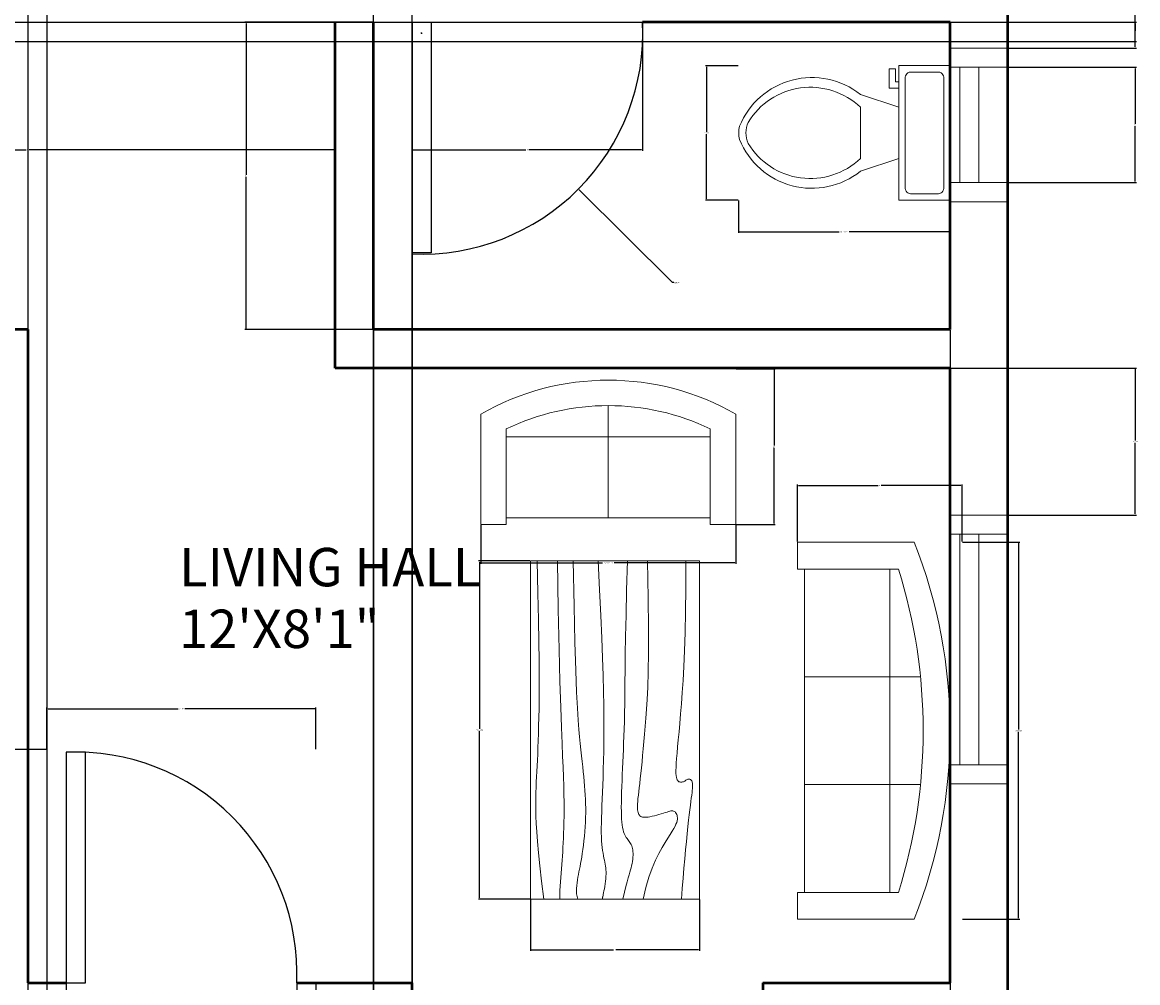
# Model space of a CAD drawing. Units: inches. Extents: x 2630 to 2982, y 643 to 1079.
# Tile 3 of 4: x 2808 to 2982, y 774 to 924. Entities that reach past the tile are written whole.
import ezdxf

# ---------------------------------------------------------------- set-up
doc = ezdxf.new("R2010")
doc.units = ezdxf.units.IN
for name, color, linetype, lineweight in [('A-ANNO-DIMS', 2, 'Continuous', 18), ('A-AREA-IDEN', 7, 'Continuous', 25), ('A-DOOR', 3, 'Continuous', 25), ('A-FLOR-FIXT', 9, 'Continuous', 18), ('A-FURN', 8, 'Continuous', 18), ('A-GLAZ', 4, 'Continuous', 18), ('A-WALL', 7, 'Continuous', 50)]:
    doc.layers.add(name, color=color, linetype=linetype, lineweight=lineweight)
doc.styles.get("Standard").update_dxf_attribs({"font": 'arial.ttf'})
doc.dimstyles.get("Standard").update_dxf_attribs({"dimtxt": 0.18, "dimasz": 0.18, "dimexe": 0.18, "dimexo": 0.0625, "dimgap": 0.09, "dimtad": 0, "dimtih": 1, "dimtoh": 1, "dimdec": 4, "dimzin": 0, "dimdsep": 46, "dimtxsty": 'Standard', "dimcen": 0.09, "dimadec": 0, "dimazin": 0, "dimtfac": 1, "dimtdec": 4, "dimtofl": 0, "dimtmove": 0, "dimatfit": 3, "dimfxl": 1, "dimtolj": 1, "dimtzin": 0, "dimarcsym": 0})

# ---------------------------------------------------------------- blocks, each defined once
blk = doc.blocks.new('Table - Rectangular Woodgrain 60 x 30 in.')
for p, q in [((0, 0), (0, -30)), ((60, 0), (0, 0)), ((60, -30), (60, 0)), ((0, -30), (60, -30))]:
    blk.add_line(p, q)
for points in [[(0, -2.4), (4.8155, -2.418), (9.0302, -2.4688), (12.709, -2.5477), (15.9167, -2.65), (18.7181, -2.7711), (21.1781, -2.9063), (23.3616, -3.0508), (25.3333, -3.2), (27.1477, -3.3495), (28.8172, -3.4958), (30.3437, -3.636), (31.7291, -3.7667), (32.9756, -3.8849), (34.0849, -3.9875), (35.059, -4.0714), (35.9, -4.1334), (36.6114, -4.1711), (37.2041, -4.1854), (37.6906, -4.1779), (38.0833, -4.15), (38.3948, -4.1034), (38.6375, -4.0396), (38.8239, -3.9602), (38.9666, -3.8667), (39.0764, -3.7608), (39.1573, -3.6448), (39.2116, -3.521), (39.2416, -3.3917), (39.2498, -3.2593), (39.2385, -3.1261), (39.21, -2.9944), (39.1666, -2.8667), (39.111, -2.7447), (39.0468, -2.6281), (38.978, -2.5163), (38.9083, -2.4083), (38.8418, -2.3035), (38.7823, -2.201), (38.7337, -2.1001), (38.7, -2), (38.6844, -1.9003), (38.6875, -1.8021), (38.7094, -1.707), (38.75, -1.6167), (38.8094, -1.5326), (38.8875, -1.4563), (38.9844, -1.3893), (39.1, -1.3333), (39.2351, -1.2896), (39.3937, -1.2583), (39.5804, -1.2396), (39.8, -1.2333), (40.057, -1.2396), (40.3562, -1.2583), (40.7023, -1.2896), (41.1, -1.3333), (41.5547, -1.3895), (42.0755, -1.4573), (42.6721, -1.5361), (43.3542, -1.625), (44.1316, -1.7233), (45.014, -1.8302), (46.0114, -1.9449), (47.1333, -2.0667), (48.3862, -2.1947), (49.7625, -2.3281), (51.2513, -2.4663), (52.8416, -2.6083), (54.5226, -2.7535), (56.2833, -2.9011), (58.1127, -3.0501), (60, -3.2)], [(0, -9.2), (6.5759, -9.0858), (11.9385, -9.0365), (16.2527, -9.0418), (19.6833, -9.0917), (22.3952, -9.1759), (24.5531, -9.2844), (26.322, -9.4069), (27.8666, -9.5333), (29.3241, -9.6553), (30.7203, -9.7719), (32.0532, -9.8837), (33.3208, -9.9917), (34.5213, -10.0965), (35.6526, -10.199), (36.7128, -10.2999), (37.7, -10.4), (38.6129, -10.4996), (39.4531, -10.5969), (40.223, -10.6895), (40.925, -10.775), (41.5613, -10.8512), (42.1344, -10.9156), (42.6465, -10.966), (43.1, -11), (43.4976, -11.0158), (43.8437, -11.0136), (44.143, -10.9942), (44.4, -10.9583), (44.6195, -10.9069), (44.8062, -10.8406), (44.9648, -10.7603), (45.1, -10.6667), (45.2155, -10.5598), (45.3114, -10.4365), (45.3871, -10.2929), (45.4416, -10.125), (45.4743, -9.929), (45.4844, -9.7011), (45.4709, -9.4371), (45.4333, -9.1333), (45.3716, -8.7883), (45.2896, -8.4104), (45.1919, -8.0107), (45.0833, -7.6), (44.9685, -7.1893), (44.8521, -6.7896), (44.7388, -6.4117), (44.6333, -6.0667), (44.54, -5.7628), (44.4614, -5.4979), (44.4001, -5.2675), (44.3583, -5.0667), (44.3384, -4.8909), (44.3427, -4.7354), (44.3736, -4.5956), (44.4333, -4.4667), (44.5236, -4.3453), (44.6427, -4.2333), (44.7884, -4.1339), (44.9583, -4.05), (45.1501, -3.9849), (45.3614, -3.9417), (45.59, -3.9234), (45.8333, -3.9333), (46.0915, -3.9749), (46.3734, -4.0531), (46.6906, -4.1736), (47.0542, -4.3417), (47.4756, -4.5629), (47.9661, -4.8427), (48.5372, -5.1866), (49.2, -5.6), (49.9676, -6.0844), (50.8594, -6.625), (51.8965, -7.2031), (53.1, -7.8), (54.491, -8.3969), (56.0906, -8.975), (57.9199, -9.5156), (60, -10)], [(0, -12.8), (5.1847, -12.9322), (9.6213, -13.0323), (13.3963, -13.1059), (16.5958, -13.1583), (19.3063, -13.1952), (21.614, -13.2219), (23.6054, -13.2439), (25.3666, -13.2667), (26.9728, -13.2947), (28.4531, -13.3281), (29.8256, -13.3663), (31.1083, -13.4083), (32.3191, -13.4535), (33.476, -13.501), (34.597, -13.5501), (35.7, -13.6), (36.7984, -13.6497), (37.8875, -13.6979), (38.9578, -13.743), (40, -13.7833), (41.0047, -13.8174), (41.9625, -13.8438), (42.864, -13.8607), (43.7, -13.8667), (44.4631, -13.8604), (45.1552, -13.8417), (45.7801, -13.8104), (46.3416, -13.7667), (46.8439, -13.7104), (47.2906, -13.6417), (47.6858, -13.5604), (48.0333, -13.4667), (48.3375, -13.3608), (48.6042, -13.2448), (48.8396, -13.121), (49.05, -12.9917), (49.2417, -12.8593), (49.4208, -12.7261), (49.5937, -12.5944), (49.7667, -12.4667), (49.9452, -12.3451), (50.1323, -12.2313), (50.3303, -12.1268), (50.5416, -12.0333), (50.7686, -11.9524), (51.0135, -11.8854), (51.2788, -11.8341), (51.5666, -11.8), (51.8785, -11.7843), (52.2116, -11.7865), (52.562, -11.8059), (52.926, -11.8417), (53.2998, -11.8931), (53.6795, -11.9594), (54.0614, -12.0397), (54.4416, -12.1333), (54.8223, -12.2401), (55.2293, -12.3625), (55.6942, -12.5037), (56.2489, -12.6667), (56.9251, -12.8547), (57.7545, -13.0708), (58.7689, -13.3182), (60, -13.6)], [(0, -18), (5.124, -17.7273), (9.6609, -17.5057), (13.6705, -17.3303), (17.2125, -17.1958), (20.3467, -17.0973), (23.1328, -17.0297), (25.6307, -16.9878), (27.9, -16.9667), (29.9928, -16.9617), (31.9302, -16.9703), (33.7254, -16.9907), (35.3917, -17.0208), (36.9423, -17.0588), (38.3906, -17.1026), (39.7499, -17.1503), (41.0333, -17.2), (42.2519, -17.2496), (43.4073, -17.2969), (44.4986, -17.3395), (45.525, -17.375), (46.4858, -17.4012), (47.3802, -17.4156), (48.2074, -17.416), (48.9667, -17.4), (49.6583, -17.3662), (50.2872, -17.3167), (50.8595, -17.2547), (51.3812, -17.1833), (51.8584, -17.1057), (52.2971, -17.025), (52.7034, -16.9443), (53.0833, -16.8667), (53.443, -16.7951), (53.789, -16.7313), (54.128, -16.6768), (54.4666, -16.6334), (54.8115, -16.6024), (55.1693, -16.5854), (55.5465, -16.5841), (55.95, -16.6), (56.3828, -16.6337), (56.8346, -16.6823), (57.2915, -16.7418), (57.7396, -16.8084), (58.165, -16.878), (58.5539, -16.9469), (58.8924, -17.0111), (59.1666, -17.0667), (59.3679, -17.1107), (59.5078, -17.1438), (59.6032, -17.1675), (59.6708, -17.1833), (59.7275, -17.193), (59.7901, -17.1979), (59.8753, -17.1998), (60, -17.2)], [(0, -22.4), (8.0098, -22.2501), (14.4094, -22.1011), (19.4168, -21.9535), (23.25, -21.8083), (26.1269, -21.6663), (28.2656, -21.5281), (29.884, -21.3947), (31.2, -21.2667), (32.3967, -21.1448), (33.5172, -21.0292), (34.5697, -20.9198), (35.5625, -20.8167), (36.5037, -20.7198), (37.4015, -20.6292), (38.2642, -20.5448), (39.1, -20.4667), (39.9164, -20.3951), (40.7187, -20.3313), (41.5117, -20.2768), (42.3, -20.2333), (43.0883, -20.2024), (43.8812, -20.1854), (44.6836, -20.1841), (45.5, -20.2), (46.3328, -20.234), (47.1747, -20.2844), (48.0163, -20.3488), (48.8479, -20.425), (49.66, -20.5106), (50.4429, -20.6031), (51.1872, -20.7004), (51.8833, -20.8), (52.5246, -20.8999), (53.1166, -20.9995), (53.6681, -21.0983), (54.1875, -21.1958), (54.6834, -21.2919), (55.1646, -21.3859), (55.6394, -21.4777), (56.1167, -21.5667), (56.6028, -21.6515), (57.0961, -21.7266), (57.5929, -21.7852), (58.0896, -21.8208), (58.5823, -21.8268), (59.0674, -21.7964), (59.5412, -21.723), (60, -21.6)], [(0, -25.2), (8.6355, -25.0504), (15.7026, -24.9031), (21.4049, -24.7606), (25.9458, -24.625), (29.529, -24.4988), (32.3578, -24.3844), (34.6359, -24.284), (36.5667, -24.2), (38.3213, -24.1341), (39.9417, -24.0854), (41.437, -24.0523), (42.8167, -24.0333), (44.0901, -24.0268), (45.2667, -24.0313), (46.3557, -24.0451), (47.3667, -24.0667), (48.309, -24.0947), (49.1928, -24.1287), (50.0284, -24.168), (50.826, -24.2125), (51.5959, -24.2617), (52.3483, -24.3151), (53.0935, -24.3725), (53.8417, -24.4334), (54.6009, -24.497), (55.3699, -24.561), (56.1454, -24.6226), (56.9239, -24.6792), (57.7021, -24.7279), (58.4764, -24.7662), (59.2435, -24.7911), (60, -24.8)], [(0, -28.8), (5.6867, -28.6681), (10.45, -28.5698), (14.407, -28.5012), (17.675, -28.4584), (20.3711, -28.4374), (22.6125, -28.4344), (24.5164, -28.4455), (26.2, -28.4667), (27.762, -28.4947), (29.2276, -28.5281), (30.6033, -28.5663), (31.8958, -28.6084), (33.1118, -28.6535), (34.2578, -28.7011), (35.3405, -28.7501), (36.3666, -28.8), (37.3443, -28.8497), (38.288, -28.8974), (39.2137, -28.9412), (40.1375, -28.9792), (41.0753, -29.0093), (42.0432, -29.0297), (43.0572, -29.0384), (44.1333, -29.0333), (45.2936, -29.0114), (46.5843, -28.9641), (48.0579, -28.8816), (49.7666, -28.7542), (51.7629, -28.5721), (54.0989, -28.3255), (56.8272, -28.0048), (60, -27.6)]]:
    blk.add_lwpolyline(points)
blk = doc.blocks.new('Sofa - Roundback Loveseat 5 ft.')
for p, q in [((0, -32.44198), (0, -5.99998)), ((-24, -33.99998), (-24, -11.46958)), ((24.00004, -33.99998), (24.00004, -11.46958)), ((-23.9998, -13.38178), (23.99986, -13.38178)), ((-24, -32.44198), (24.00004, -32.44198))]:
    blk.add_line(p, q)
for points in [[(-24, -33.99998), (-30, -33.99998), (-30, -7.99998)], [(30.00004, -7.99998), (30.00004, -33.99998), (24.00004, -33.99998)]]:
    blk.add_lwpolyline(points)
for centre, radius, start, end in [((0, -60.24998), 60.24998, 60.13715, 119.8628), ((0, -61.38438), 55.38444, 64.32083, 115.6792)]:
    blk.add_arc(centre, radius, start, end)
blk = doc.blocks.new('Sofa - Roundback 7 ft.')
for p, q in [((-12.00002, -32.4421), (-12.00003, -6.5971)), ((11.99997, -32.4421), (11.99998, -6.5971)), ((-36.000027, -34), (-36.000027, -11.4696)), ((35.99998, -34), (35.99998, -11.4696)), ((-35.999844, -13.3819), (35.9998, -13.3819)), ((-36.000027, -32.4421), (35.99998, -32.4421))]:
    blk.add_line(p, q)
for points in [[(-36.000027, -34), (-42.000027, -34), (-42.000027, -8)], [(41.99998, -8), (41.99998, -34), (35.99998, -34)]]:
    blk.add_lwpolyline(points)
for centre, radius, start, end in [((0, -114.25), 114.25, 68.43141, 111.5686), ((-0.00001, -127.1968), 121.1968, 72.72033, 107.2797)]:
    blk.add_arc(centre, radius, start, end)
blk = doc.blocks.new('Toilet - top')
for p, q in [((9.5, -6), (9.5, -2)), ((-10, -8.5), (-8, -8.5)), ((-10, -9.5), (-10, -8.5)), ((-8, -8.5), (-8, -8)), ((-7, -8), (-7, -9.5)), ((-4, -8), (-6, -14)), ((4, -8), (6, -14)), ((-7, -9.5), (-10, -9.5)), ((4, -14), (-4, -14))]:
    blk.add_line(p, q)
blk.add_lwpolyline([(10.5, -8), (10.5, 0), (-10.5, 0), (-10.5, -8)], close=True)
for points in [[(8.5, -1), (-8.5, -1)], [(-9.5, -2), (-9.5, -6)], [(-8.5, -7), (8.5, -7)]]:
    blk.add_lwpolyline(points)
for centre, radius, start, end in [((-8.62, -1.88), 0.884, 81.8699, 188.1301), ((8.62, -1.88), 0.884, 351.8699, 98.1301), ((-8.62, -6.12), 0.884, 171.8699, 278.1301), ((8.62, -6.12), 0.884, 261.8699, 8.1301), ((3.52, -21.58), 12.17, 141.4691, 247.9714), ((4.2, -21.82), 11.33, 136.3677, 238.9468), ((-3.52, -21.58), 12.17, 292.0284, 38.5307), ((-4.2, -21.82), 11.33, 301.053, 43.6321), ((0, -27.88), 4, 245.7318, 294.2682), ((0, -29), 4, 254.8605, 285.1395)]:
    blk.add_arc(centre, radius, start, end)
blk = doc.blocks.new('DOOR-36IN-INT')
for p, q in [((0, 6), (0, 0)), ((3, 6), (3, 0)), ((39, 6), (39, 0)), ((42, 6), (42, 0))]:
    blk.add_line(p, q)
blk.add_lwpolyline([(3, 6), (6, 6), (6, 42), (3, 42)], close=True)
blk.add_arc((4.5, 7.5), 34.53, 357.5104, 92.4896)
blk = doc.blocks.new('WIN-36IN')
for p, q in [((9, 42), (0, 42)), ((9, 39), (0, 39)), ((4.5, 3), (4.5, 39)), ((7.5, 3), (7.5, 39)), ((0, 3), (9, 3)), ((0, 0), (9, 0))]:
    blk.add_line(p, q)
blk = doc.blocks.new('WIN-18IN')
for p, q in [((9, 24), (0, 24)), ((9, 21), (0, 21)), ((1.5, 21), (1.5, 3)), ((4.5, 21), (4.5, 3)), ((0, 3), (9, 3)), ((0, 0), (9, 0))]:
    blk.add_line(p, q)
blk = doc.blocks.new('*D19')
at = {"layer": 'A-ANNO-DIMS', "color": 0, "lineweight": -2, "transparency": 16777216}
for p, q in [((2811.7, 810.29), (2805.22, 810.29)), ((2805.4, 810.11), (2805.4, 789.26)), ((2805.4, 768.05), (2805.4, 788.89)), ((2811.7, 767.87), (2805.22, 767.87))]:
    blk.add_line(p, q, dxfattribs=at)
at = {"layer": 'A-ANNO-DIMS', "color": 0, "transparency": 16777216}
for points in [[(2805.37, 810.11), (2805.43, 810.11), (2805.4, 810.29)], [(2805.37, 768.05), (2805.43, 768.05), (2805.4, 767.87)]]:
    blk.add_solid(points, dxfattribs=at)
at = {"layer": 'Defpoints', "color": 0, "transparency": 16777216}
for p in [(2805.4, 810.29), (2811.77, 810.29), (2811.77, 767.87)]:
    blk.add_point(p, dxfattribs=at)
at = {"layer": 'A-ANNO-DIMS', "color": 0, "transparency": 16777216, "insert": (2805.4, 789.08), "char_height": 0.18, "attachment_point": 5}
blk.add_mtext('\\A1;DOOR D1 42 TYP.', dxfattribs=at)
blk = doc.blocks.new('*D20')
at = {"layer": 'A-ANNO-DIMS', "color": 0, "lineweight": -2, "transparency": 16777216}
for p, q in [((2811.77, 810.35), (2811.77, 816.83)), ((2811.95, 816.65), (2832.24, 816.65)), ((2853.59, 816.65), (2833.3, 816.65)), ((2853.77, 810.35), (2853.77, 816.83))]:
    blk.add_line(p, q, dxfattribs=at)
at = {"layer": 'A-ANNO-DIMS', "color": 0, "transparency": 16777216}
for points in [[(2811.95, 816.68), (2811.95, 816.62), (2811.77, 816.65)], [(2853.59, 816.68), (2853.59, 816.62), (2853.77, 816.65)]]:
    blk.add_solid(points, dxfattribs=at)
at = {"layer": 'Defpoints', "color": 0, "transparency": 16777216}
for p in [(2853.77, 816.65), (2811.77, 810.29), (2853.77, 810.29)]:
    blk.add_point(p, dxfattribs=at)
at = {"layer": 'A-ANNO-DIMS', "color": 0, "transparency": 16777216, "insert": (2832.77, 816.65), "char_height": 0.18, "attachment_point": 5}
blk.add_mtext('\\A1;42 TYP.', dxfattribs=at)
blk = doc.blocks.new('*D21')
at = {"layer": 'A-ANNO-DIMS', "color": 0, "lineweight": -2, "transparency": 16777216}
for p, q in [((2919.72, 896.03), (2919.72, 890.96)), ((2952.77, 896.03), (2952.77, 890.96)), ((2919.9, 891.14), (2935.47, 891.14)), ((2952.59, 891.14), (2937.02, 891.14))]:
    blk.add_line(p, q, dxfattribs=at)
at = {"layer": 'A-ANNO-DIMS', "color": 0, "transparency": 16777216}
for points in [[(2919.9, 891.17), (2919.9, 891.11), (2919.72, 891.14)], [(2952.59, 891.17), (2952.59, 891.11), (2952.77, 891.14)]]:
    blk.add_solid(points, dxfattribs=at)
at = {"layer": 'Defpoints', "color": 0, "transparency": 16777216}
for p in [(2919.72, 896.09), (2952.77, 896.09), (2952.77, 891.14)]:
    blk.add_point(p, dxfattribs=at)
at = {"layer": 'A-ANNO-DIMS', "color": 0, "transparency": 16777216, "insert": (2936.24, 891.14), "char_height": 0.18, "attachment_point": 5}
blk.add_mtext('\\A1;WC 33 TYP.', dxfattribs=at)
blk = doc.blocks.new('*D22')
at = {"layer": 'A-ANNO-DIMS', "color": 0, "lineweight": -2, "transparency": 16777216}
for p, q in [((2919.66, 917.09), (2914.58, 917.09)), ((2914.76, 916.91), (2914.76, 906.77)), ((2914.76, 896.27), (2914.76, 906.41)), ((2919.66, 896.09), (2914.58, 896.09))]:
    blk.add_line(p, q, dxfattribs=at)
at = {"layer": 'A-ANNO-DIMS', "color": 0, "transparency": 16777216}
for points in [[(2914.73, 916.91), (2914.79, 916.91), (2914.76, 917.09)], [(2914.73, 896.27), (2914.79, 896.27), (2914.76, 896.09)]]:
    blk.add_solid(points, dxfattribs=at)
at = {"layer": 'Defpoints', "color": 0, "transparency": 16777216}
for p in [(2919.72, 917.09), (2914.76, 896.09), (2919.72, 896.09)]:
    blk.add_point(p, dxfattribs=at)
at = {"layer": 'A-ANNO-DIMS', "color": 0, "transparency": 16777216, "insert": (2914.76, 906.59), "char_height": 0.18, "attachment_point": 5}
blk.add_mtext('\\A1;21 TYP.', dxfattribs=at)
blk = doc.blocks.new('*D29')
at = {"layer": 'A-ANNO-DIMS', "color": 0, "lineweight": -2, "transparency": 16777216}
for p, q in [((2887.18, 839.73), (2879.14, 839.73)), ((2879.32, 839.55), (2879.32, 813.51)), ((2879.32, 787.1), (2879.32, 813.14)), ((2887.18, 786.92), (2879.14, 786.92))]:
    blk.add_line(p, q, dxfattribs=at)
at = {"layer": 'A-ANNO-DIMS', "color": 0, "transparency": 16777216}
for points in [[(2879.29, 839.55), (2879.35, 839.55), (2879.32, 839.73)], [(2879.29, 787.1), (2879.35, 787.1), (2879.32, 786.92)]]:
    blk.add_solid(points, dxfattribs=at)
at = {"layer": 'Defpoints', "color": 0, "transparency": 16777216}
for p in [(2887.24, 839.73), (2879.32, 786.92), (2887.24, 786.92)]:
    blk.add_point(p, dxfattribs=at)
at = {"layer": 'A-ANNO-DIMS', "color": 0, "transparency": 16777216, "insert": (2879.32, 813.33), "char_height": 0.18, "attachment_point": 5}
blk.add_mtext('\\A1;TABLE 53', dxfattribs=at)
blk = doc.blocks.new('*D30')
at = {"layer": 'A-ANNO-DIMS', "color": 0, "lineweight": -2, "transparency": 16777216}
for p, q in [((2887.24, 786.86), (2887.24, 778.82)), ((2913.65, 786.86), (2913.65, 778.82)), ((2887.42, 779), (2900.22, 779)), ((2913.47, 779), (2900.66, 779))]:
    blk.add_line(p, q, dxfattribs=at)
at = {"layer": 'A-ANNO-DIMS', "color": 0, "transparency": 16777216}
for points in [[(2887.42, 779.03), (2887.42, 778.97), (2887.24, 779)], [(2913.47, 779.03), (2913.47, 778.97), (2913.65, 779)]]:
    blk.add_solid(points, dxfattribs=at)
at = {"layer": 'Defpoints', "color": 0, "transparency": 16777216}
for p in [(2887.24, 786.92), (2913.65, 786.92), (2913.65, 779)]:
    blk.add_point(p, dxfattribs=at)
at = {"layer": 'A-ANNO-DIMS', "color": 0, "transparency": 16777216, "insert": (2900.44, 779), "char_height": 0.18, "attachment_point": 5}
blk.add_mtext('\\A1;26', dxfattribs=at)
blk = doc.blocks.new('*D31')
at = {"layer": 'A-ANNO-DIMS', "color": 0, "lineweight": -2, "transparency": 16777216}
for p, q in [((2879.5, 845.35), (2879.5, 839.27)), ((2919.32, 845.35), (2919.32, 839.27)), ((2879.68, 839.45), (2898.5, 839.45)), ((2919.14, 839.45), (2900.32, 839.45))]:
    blk.add_line(p, q, dxfattribs=at)
at = {"layer": 'A-ANNO-DIMS', "color": 0, "transparency": 16777216}
for points in [[(2879.68, 839.48), (2879.68, 839.42), (2879.5, 839.45)], [(2919.14, 839.48), (2919.14, 839.42), (2919.32, 839.45)]]:
    blk.add_solid(points, dxfattribs=at)
at = {"layer": 'Defpoints', "color": 0, "transparency": 16777216}
for p in [(2879.5, 845.42), (2919.32, 845.42), (2919.32, 839.45)]:
    blk.add_point(p, dxfattribs=at)
at = {"layer": 'A-ANNO-DIMS', "color": 0, "transparency": 16777216, "insert": (2899.41, 839.45), "char_height": 0.18, "attachment_point": 5}
blk.add_mtext('\\A1;LOVESEAT 40', dxfattribs=at)
blk = doc.blocks.new('*D32')
at = {"layer": 'A-ANNO-DIMS', "color": 0, "lineweight": -2, "transparency": 16777216}
for p, q in [((2919.38, 869.75), (2925.47, 869.75)), ((2925.29, 869.57), (2925.29, 857.76)), ((2925.29, 845.6), (2925.29, 857.4)), ((2919.38, 845.42), (2925.47, 845.42))]:
    blk.add_line(p, q, dxfattribs=at)
at = {"layer": 'A-ANNO-DIMS', "color": 0, "transparency": 16777216}
for points in [[(2925.26, 869.57), (2925.32, 869.57), (2925.29, 869.75)], [(2925.26, 845.6), (2925.32, 845.6), (2925.29, 845.42)]]:
    blk.add_solid(points, dxfattribs=at)
at = {"layer": 'Defpoints', "color": 0, "transparency": 16777216}
for p in [(2919.32, 869.75), (2925.29, 869.75), (2919.32, 845.42)]:
    blk.add_point(p, dxfattribs=at)
at = {"layer": 'A-ANNO-DIMS', "color": 0, "transparency": 16777216, "insert": (2925.29, 857.58), "char_height": 0.18, "attachment_point": 5}
blk.add_mtext('\\A1;24', dxfattribs=at)
blk = doc.blocks.new('*D33')
at = {"layer": 'A-ANNO-DIMS', "color": 0, "lineweight": -2, "transparency": 16777216}
for p, q in [((2954.7, 842.68), (2963.65, 842.68)), ((2963.47, 842.5), (2963.47, 813.41)), ((2963.47, 783.95), (2963.47, 813.04)), ((2954.7, 783.77), (2963.65, 783.77))]:
    blk.add_line(p, q, dxfattribs=at)
at = {"layer": 'A-ANNO-DIMS', "color": 0, "transparency": 16777216}
for points in [[(2963.44, 842.5), (2963.5, 842.5), (2963.47, 842.68)], [(2963.44, 783.95), (2963.5, 783.95), (2963.47, 783.77)]]:
    blk.add_solid(points, dxfattribs=at)
at = {"layer": 'Defpoints', "color": 0, "transparency": 16777216}
for p in [(2954.64, 842.68), (2954.64, 783.77), (2963.47, 783.77)]:
    blk.add_point(p, dxfattribs=at)
at = {"layer": 'A-ANNO-DIMS', "color": 0, "transparency": 16777216, "insert": (2963.47, 813.23), "char_height": 0.18, "attachment_point": 5}
blk.add_mtext('\\A1;SOFA 59', dxfattribs=at)
blk = doc.blocks.new('*D34')
at = {"layer": 'A-ANNO-DIMS', "color": 0, "lineweight": -2, "transparency": 16777216}
for p, q in [((2928.92, 842.75), (2928.92, 851.7)), ((2929.1, 851.52), (2941.56, 851.52)), ((2954.46, 851.52), (2942, 851.52)), ((2954.64, 842.75), (2954.64, 851.7))]:
    blk.add_line(p, q, dxfattribs=at)
at = {"layer": 'A-ANNO-DIMS', "color": 0, "transparency": 16777216}
for points in [[(2929.1, 851.55), (2929.1, 851.49), (2928.92, 851.52)], [(2954.46, 851.55), (2954.46, 851.49), (2954.64, 851.52)]]:
    blk.add_solid(points, dxfattribs=at)
at = {"layer": 'Defpoints', "color": 0, "transparency": 16777216}
for p in [(2954.64, 851.52), (2928.92, 842.68), (2954.64, 842.68)]:
    blk.add_point(p, dxfattribs=at)
at = {"layer": 'A-ANNO-DIMS', "color": 0, "transparency": 16777216, "insert": (2941.78, 851.52), "char_height": 0.18, "attachment_point": 5}
blk.add_mtext('\\A1;26', dxfattribs=at)
blk = doc.blocks.new('*D46')
at = {"layer": 'A-ANNO-DIMS', "color": 0, "lineweight": -2, "transparency": 16777216}
for p, q in [((2961.83, 970.69), (2981.86, 970.69)), ((2981.68, 970.51), (2981.68, 945.45)), ((2981.68, 920.02), (2981.68, 945.08)), ((2961.83, 919.84), (2981.86, 919.84))]:
    blk.add_line(p, q, dxfattribs=at)
at = {"layer": 'A-ANNO-DIMS', "color": 0, "transparency": 16777216}
for points in [[(2981.65, 970.51), (2981.71, 970.51), (2981.68, 970.69)], [(2981.65, 920.02), (2981.71, 920.02), (2981.68, 919.84)]]:
    blk.add_solid(points, dxfattribs=at)
at = {"layer": 'Defpoints', "color": 0, "transparency": 16777216}
for p in [(2961.77, 970.69), (2981.68, 970.69), (2961.77, 919.84)]:
    blk.add_point(p, dxfattribs=at)
at = {"layer": 'A-ANNO-DIMS', "color": 0, "transparency": 16777216, "insert": (2981.68, 945.27), "char_height": 0.18, "attachment_point": 5}
blk.add_mtext('\\A1;50.85', dxfattribs=at)
blk = doc.blocks.new('*D47')
at = {"layer": 'A-ANNO-DIMS', "color": 0, "lineweight": -2, "transparency": 16777216}
for p, q in [((2952.83, 869.87), (2981.86, 869.87)), ((2981.68, 869.69), (2981.68, 858.57)), ((2981.68, 847.09), (2981.68, 858.21)), ((2961.83, 846.91), (2981.86, 846.91))]:
    blk.add_line(p, q, dxfattribs=at)
at = {"layer": 'A-ANNO-DIMS', "color": 0, "transparency": 16777216}
for points in [[(2981.65, 869.69), (2981.71, 869.69), (2981.68, 869.87)], [(2981.65, 847.09), (2981.71, 847.09), (2981.68, 846.91)]]:
    blk.add_solid(points, dxfattribs=at)
at = {"layer": 'Defpoints', "color": 0, "transparency": 16777216}
for p in [(2952.77, 869.87), (2981.68, 869.87), (2961.77, 846.91)]:
    blk.add_point(p, dxfattribs=at)
at = {"layer": 'A-ANNO-DIMS', "color": 0, "transparency": 16777216, "insert": (2981.68, 858.39), "char_height": 0.18, "attachment_point": 5}
blk.add_mtext('\\A1;22.954', dxfattribs=at)
blk = doc.blocks.new('*D51')
at = {"layer": 'A-ANNO-DIMS', "color": 0, "lineweight": -2, "transparency": 16777216}
for p, q in [((2862.77, 875.8), (2862.77, 642.78)), ((2952.77, 875.8), (2952.77, 642.78)), ((2862.95, 642.96), (2907.55, 642.96)), ((2952.59, 642.96), (2907.99, 642.96))]:
    blk.add_line(p, q, dxfattribs=at)
at = {"layer": 'A-ANNO-DIMS', "color": 0, "transparency": 16777216}
for points in [[(2862.95, 642.99), (2862.95, 642.93), (2862.77, 642.96)], [(2952.59, 642.99), (2952.59, 642.93), (2952.77, 642.96)]]:
    blk.add_solid(points, dxfattribs=at)
at = {"layer": 'Defpoints', "color": 0, "transparency": 16777216}
for p in [(2862.77, 875.87), (2952.77, 875.87), (2952.77, 642.96)]:
    blk.add_point(p, dxfattribs=at)
at = {"layer": 'A-ANNO-DIMS', "color": 0, "transparency": 16777216, "insert": (2907.77, 642.96), "char_height": 0.18, "attachment_point": 5}
blk.add_mtext('\\A1;90', dxfattribs=at)
blk = doc.blocks.new('*D52')
at = {"layer": 'A-ANNO-DIMS', "color": 0, "lineweight": -2, "transparency": 16777216}
for p, q in [((2862.7, 923.87), (2842.68, 923.87)), ((2842.86, 923.69), (2842.86, 900.05)), ((2842.86, 876.05), (2842.86, 899.68)), ((2862.7, 875.87), (2842.68, 875.87))]:
    blk.add_line(p, q, dxfattribs=at)
at = {"layer": 'A-ANNO-DIMS', "color": 0, "transparency": 16777216}
for points in [[(2842.83, 923.69), (2842.89, 923.69), (2842.86, 923.87)], [(2842.83, 876.05), (2842.89, 876.05), (2842.86, 875.87)]]:
    blk.add_solid(points, dxfattribs=at)
at = {"layer": 'Defpoints', "color": 0, "transparency": 16777216}
for p in [(2842.86, 923.87), (2862.77, 923.87), (2862.77, 875.87)]:
    blk.add_point(p, dxfattribs=at)
at = {"layer": 'A-ANNO-DIMS', "color": 0, "transparency": 16777216, "insert": (2842.86, 899.87), "char_height": 0.18, "attachment_point": 5}
blk.add_mtext('\\A1;48', dxfattribs=at)
blk = doc.blocks.new('*D58')
at = {"layer": 'A-ANNO-DIMS', "color": 0, "lineweight": -2, "transparency": 16777216}
for p, q in [((2862.77, 767.93), (2862.77, 1078.96)), ((2862.95, 1078.78), (2865.62, 1078.78)), ((2868.59, 1078.78), (2865.92, 1078.78)), ((2868.77, 767.93), (2868.77, 1078.96))]:
    blk.add_line(p, q, dxfattribs=at)
at = {"layer": 'A-ANNO-DIMS', "color": 0, "transparency": 16777216}
for points in [[(2862.95, 1078.81), (2862.95, 1078.75), (2862.77, 1078.78)], [(2868.59, 1078.81), (2868.59, 1078.75), (2868.77, 1078.78)]]:
    blk.add_solid(points, dxfattribs=at)
at = {"layer": 'Defpoints', "color": 0, "transparency": 16777216}
for p in [(2868.77, 1078.78), (2862.77, 767.87), (2868.77, 767.87)]:
    blk.add_point(p, dxfattribs=at)
at = {"layer": 'A-ANNO-DIMS', "color": 0, "transparency": 16777216, "insert": (2865.77, 1078.78), "char_height": 0.18, "attachment_point": 5}
blk.add_mtext('\\A1;6', dxfattribs=at)
blk = doc.blocks.new('*D59')
at = {"layer": 'A-ANNO-DIMS', "color": 0, "lineweight": -2, "transparency": 16777216}
for p, q in [((2808.77, 929.8), (2808.77, 642.78)), ((2811.77, 929.8), (2811.77, 642.78)), ((2808.95, 642.96), (2810.12, 642.96)), ((2811.59, 642.96), (2810.42, 642.96))]:
    blk.add_line(p, q, dxfattribs=at)
at = {"layer": 'A-ANNO-DIMS', "color": 0, "transparency": 16777216}
for points in [[(2808.95, 642.99), (2808.95, 642.93), (2808.77, 642.96)], [(2811.59, 642.99), (2811.59, 642.93), (2811.77, 642.96)]]:
    blk.add_solid(points, dxfattribs=at)
at = {"layer": 'Defpoints', "color": 0, "transparency": 16777216}
for p in [(2808.77, 929.87), (2811.77, 929.87), (2811.77, 642.96)]:
    blk.add_point(p, dxfattribs=at)
at = {"layer": 'A-ANNO-DIMS', "color": 0, "transparency": 16777216, "insert": (2810.27, 642.96), "char_height": 0.18, "attachment_point": 5}
blk.add_mtext('\\A1;3', dxfattribs=at)
blk = doc.blocks.new('*D60')
at = {"layer": 'A-ANNO-DIMS', "color": 0, "lineweight": -2, "transparency": 16777216}
for p, q in [((2862.77, 923.8), (2862.77, 642.78)), ((2868.77, 923.8), (2868.77, 642.78)), ((2862.95, 642.96), (2865.62, 642.96)), ((2868.59, 642.96), (2865.92, 642.96))]:
    blk.add_line(p, q, dxfattribs=at)
at = {"layer": 'A-ANNO-DIMS', "color": 0, "transparency": 16777216}
for points in [[(2862.95, 642.99), (2862.95, 642.93), (2862.77, 642.96)], [(2868.59, 642.99), (2868.59, 642.93), (2868.77, 642.96)]]:
    blk.add_solid(points, dxfattribs=at)
at = {"layer": 'Defpoints', "color": 0, "transparency": 16777216}
for p in [(2862.77, 923.87), (2868.77, 923.87), (2868.77, 642.96)]:
    blk.add_point(p, dxfattribs=at)
at = {"layer": 'A-ANNO-DIMS', "color": 0, "transparency": 16777216, "insert": (2865.77, 642.96), "char_height": 0.18, "attachment_point": 5}
blk.add_mtext('\\A1;6', dxfattribs=at)
blk = doc.blocks.new('*D61')
at = {"layer": 'A-ANNO-DIMS', "color": 0, "lineweight": -2, "transparency": 16777216}
for p, q in [((2754.83, 923.87), (2981.86, 923.87)), ((2981.68, 923.69), (2981.68, 922.55)), ((2981.68, 921.05), (2981.68, 922.18)), ((2754.83, 920.87), (2981.86, 920.87))]:
    blk.add_line(p, q, dxfattribs=at)
at = {"layer": 'A-ANNO-DIMS', "color": 0, "transparency": 16777216}
for points in [[(2981.65, 923.69), (2981.71, 923.69), (2981.68, 923.87)], [(2981.65, 921.05), (2981.71, 921.05), (2981.68, 920.87)]]:
    blk.add_solid(points, dxfattribs=at)
at = {"layer": 'Defpoints', "color": 0, "transparency": 16777216}
for p in [(2754.77, 923.87), (2754.77, 920.87), (2981.68, 920.87)]:
    blk.add_point(p, dxfattribs=at)
at = {"layer": 'A-ANNO-DIMS', "color": 0, "transparency": 16777216, "insert": (2981.68, 922.37), "char_height": 0.18, "attachment_point": 5}
blk.add_mtext('\\A1;3', dxfattribs=at)
blk = doc.blocks.new('*D63')
at = {"layer": 'A-ANNO-DIMS', "color": 0, "lineweight": -2, "transparency": 16777216}
for p, q in [((2868.77, 923.8), (2868.77, 903.78)), ((2904.77, 923.8), (2904.77, 903.78)), ((2868.95, 903.96), (2886.55, 903.96)), ((2904.59, 903.96), (2886.99, 903.96))]:
    blk.add_line(p, q, dxfattribs=at)
at = {"layer": 'A-ANNO-DIMS', "color": 0, "transparency": 16777216}
for points in [[(2868.95, 903.99), (2868.95, 903.93), (2868.77, 903.96)], [(2904.59, 903.99), (2904.59, 903.93), (2904.77, 903.96)]]:
    blk.add_solid(points, dxfattribs=at)
at = {"layer": 'Defpoints', "color": 0, "transparency": 16777216}
for p in [(2868.77, 923.87), (2904.77, 923.87), (2868.77, 903.96)]:
    blk.add_point(p, dxfattribs=at)
at = {"layer": 'A-ANNO-DIMS', "color": 0, "transparency": 16777216, "insert": (2886.77, 903.96), "char_height": 0.18, "attachment_point": 5}
blk.add_mtext('\\A1;36', dxfattribs=at)
blk = doc.blocks.new('*D64')
at = {"layer": 'A-ANNO-DIMS', "color": 0, "lineweight": -2, "transparency": 16777216}
for p, q in [((2760.77, 923.8), (2760.77, 903.78)), ((2856.77, 923.8), (2856.77, 903.78)), ((2760.95, 903.96), (2808.55, 903.96)), ((2856.59, 903.96), (2808.99, 903.96))]:
    blk.add_line(p, q, dxfattribs=at)
at = {"layer": 'A-ANNO-DIMS', "color": 0, "transparency": 16777216}
for points in [[(2760.95, 903.99), (2760.95, 903.93), (2760.77, 903.96)], [(2856.59, 903.99), (2856.59, 903.93), (2856.77, 903.96)]]:
    blk.add_solid(points, dxfattribs=at)
at = {"layer": 'Defpoints', "color": 0, "transparency": 16777216}
for p in [(2760.77, 923.87), (2856.77, 923.87), (2760.77, 903.96)]:
    blk.add_point(p, dxfattribs=at)
at = {"layer": 'A-ANNO-DIMS', "color": 0, "transparency": 16777216, "insert": (2808.77, 903.96), "char_height": 0.18, "attachment_point": 5}
blk.add_mtext('\\A1;96', dxfattribs=at)
blk = doc.blocks.new('*D67')
at = {"layer": 'A-ANNO-DIMS', "color": 0, "lineweight": -2, "transparency": 16777216}
for p, q in [((2961.83, 916.84), (2981.86, 916.84)), ((2981.68, 916.66), (2981.68, 908.02)), ((2981.68, 899.02), (2981.68, 907.66)), ((2961.83, 898.84), (2981.86, 898.84))]:
    blk.add_line(p, q, dxfattribs=at)
at = {"layer": 'A-ANNO-DIMS', "color": 0, "transparency": 16777216}
for points in [[(2981.65, 916.66), (2981.71, 916.66), (2981.68, 916.84)], [(2981.65, 899.02), (2981.71, 899.02), (2981.68, 898.84)]]:
    blk.add_solid(points, dxfattribs=at)
at = {"layer": 'Defpoints', "color": 0, "transparency": 16777216}
for p in [(2961.77, 916.84), (2961.77, 898.84), (2981.68, 898.84)]:
    blk.add_point(p, dxfattribs=at)
at = {"layer": 'A-ANNO-DIMS', "color": 0, "transparency": 16777216, "insert": (2981.68, 907.84), "char_height": 0.18, "attachment_point": 5}
blk.add_mtext('\\A1;18', dxfattribs=at)
blk = doc.blocks.new('*D70')
at = {"layer": 'A-ANNO-DIMS', "color": 0, "lineweight": -2, "transparency": 16777216}
for p, q in [((2870.18, 922.19), (2870.36, 922.19)), ((2870.27, 922.1), (2870.27, 922.28)), ((2909.44, 883.21), (2894.88, 897.7)), ((2909.62, 883.21), (2909.44, 883.21))]:
    blk.add_line(p, q, dxfattribs=at)
at = {"layer": 'A-ANNO-DIMS', "color": 0, "transparency": 16777216}
blk.add_solid([(2894.9, 897.73), (2894.86, 897.68), (2894.75, 897.83)], dxfattribs=at)
at = {"layer": 'Defpoints', "color": 0, "transparency": 16777216}
for p in [(2870.27, 922.19), (2894.75, 897.83)]:
    blk.add_point(p, dxfattribs=at)
at = {"layer": 'A-ANNO-DIMS', "color": 0, "transparency": 16777216, "insert": (2910.1, 883.21), "char_height": 0.18, "attachment_point": 5}
blk.add_mtext('\\A1;R34.54', dxfattribs=at)

msp = doc.modelspace()

# ---------------------------------------------------------------- linework, layer by layer
at = {"layer": 'A-DOOR'}
msp.add_lwpolyline([(2868.7671, 923.8666), (2871.7671, 923.8666), (2871.7671, 887.8666), (2868.7671, 887.8666)], close=True, dxfattribs=at)
msp.add_arc((2870.2671, 922.1944), 34.5405, 267.511018, 2.775059, dxfattribs=at)
at = {"layer": 'A-WALL'}
for p, q in [((2856.7671, 869.8666), (2856.7671, 923.8666)), ((2862.7671, 875.8666), (2862.7671, 923.8666)), ((2952.7671, 923.8666), (2904.7671, 923.8666)), ((2952.7671, 875.8666), (2952.7671, 923.8666)), ((2808.7671, 875.8666), (2796.7671, 875.8666)), ((2808.7671, 875.8666), (2808.7671, 773.8666)), ((2952.7671, 875.8666), (2862.7671, 875.8666)), ((2952.7671, 869.8666), (2856.7671, 869.8666)), ((2952.7671, 773.8666), (2952.7671, 869.8666)), ((2808.7671, 773.8666), (2814.7671, 773.8666)), ((2850.7671, 773.8666), (2868.7671, 773.8666)), ((2868.7671, 767.8666), (2868.7671, 773.8666)), ((2923.557, 773.8666), (2952.7671, 773.8666)), ((2923.557, 773.8666), (2923.557, 767.8666))]:
    msp.add_line(p, q, dxfattribs=at)
msp.add_lwpolyline([(2850.7671, 662.8666), (2961.7671, 662.8666), (2961.7671, 1058.8666), (2649.7671, 1058.8666), (2649.7671, 662.8666), (2814.7671, 662.8666)], dxfattribs=at)

# ---------------------------------------------------------------- block references
at = {"layer": 'A-DOOR'}
msp.add_blockref('DOOR-36IN-INT', (2811.767, 767.867), dxfattribs=at)
at = {"layer": 'A-FLOR-FIXT', "rotation": 270}
msp.add_blockref('Toilet - top', (2952.7671, 906.5932), dxfattribs=at)
at = {"layer": 'A-FURN', "xscale": 0.6635448158332695, "yscale": 0.6635448158332695, "zscale": 0.6635448158332695}
msp.add_blockref('Sofa - Roundback Loveseat 5 ft.', (2899.409, 867.9775), dxfattribs=at)
at = {"layer": 'A-FURN', "rotation": 270}
for name, p, xscale, yscale, zscale in [('Sofa - Roundback 7 ft.', (2952.7671, 813.2252), 0.7013724099311335, 0.7013724099311335, 0.7013724099311335), ('Table - Rectangular Woodgrain 60 x 30 in.', (2913.6484, 839.7342), 0.8802759729068439, 0.8802759729068439, 0.8802759729068439)]:
    msp.add_blockref(name, p, dxfattribs=dict(at, xscale=xscale, yscale=yscale, zscale=zscale))
at = {"layer": 'A-GLAZ'}
msp.add_blockref('WIN-18IN', (2952.767, 895.843), dxfattribs=at)
at = {"layer": 'A-GLAZ', "rotation": 180}
msp.add_blockref('WIN-36IN', (2961.7672, 846.9129), dxfattribs=at)

# ---------------------------------------------------------------- texts
at = {"layer": 'A-AREA-IDEN'}
for s, p in [('LIVING HALL', (2832.41, 835.7745)), ('12\'X8\'1"', (2832.41, 826.136))]:
    msp.add_text(s, height=6, dxfattribs=at).set_placement(p)

# ---------------------------------------------------------------- dimensions: what is measured, and where the dimension line sits
at = {"layer": 'A-ANNO-DIMS'}
for base, p1, p2, picture, middle in [((2868.7671, 1078.7766), (2862.7671, 767.8666), (2868.7671, 767.8666), '*D58', (2865.7671, 1078.7766)), ((2811.7671, 642.9566), (2808.7671, 929.8666), (2811.7671, 929.8666), '*D59', (2810.2671, 642.9566)), ((2868.7671, 642.9566), (2862.7671, 923.8666), (2868.7671, 923.8666), '*D60', (2865.7671, 642.9566)), ((2952.7671, 642.9566), (2862.7671, 875.8666), (2952.7671, 875.8666), '*D51', (2907.7671, 642.9566)), ((2954.6374, 851.5202), (2928.9204, 842.6829), (2954.6374, 842.6829), '*D34', (2941.7789, 851.5202)), ((2913.6484, 778.9951), (2887.2401, 786.9176), (2913.6484, 786.9176), '*D30', (2900.4443, 778.9951))]:
    dim = msp.add_linear_dim(base=base, p1=p1, p2=p2, dimstyle='Standard', override={"dimdec": 0, "dimlfac": 1, "dimrnd": 0, "dimzin": 0, "dimdsep": 46, "dimlunit": 2}, dxfattribs=at)
    dim.commit()
    dim.dimension.update_dxf_attribs({"geometry": picture, "text_midpoint": middle})
for base, p1, p2, angle, override, picture, middle in [((2981.6771, 970.6885), (2961.7671, 919.8429), (2961.7671, 970.6885), 90, {"dimdec": 2, "dimlfac": 1, "dimrnd": 0, "dimzin": 0, "dimdsep": 46, "dimlunit": 2}, '*D46', (2981.6771, 945.2657)), ((2981.6771, 920.8666), (2754.7671, 923.8666), (2754.7671, 920.8666), 90, {"dimdec": 0, "dimlfac": 1, "dimrnd": 0, "dimzin": 0, "dimdsep": 46, "dimlunit": 2}, '*D61', (2981.6771, 922.3666)), ((2760.7671, 903.9566), (2856.7671, 923.8666), (2760.7671, 923.8666), 180, {"dimdec": 0, "dimlfac": 1, "dimrnd": 0, "dimzin": 0, "dimdsep": 46, "dimlunit": 2}, '*D64', (2808.7671, 903.9566)), ((2842.8571, 923.8666), (2862.7671, 875.8666), (2862.7671, 923.8666), 90, {"dimdec": 0, "dimlfac": 1, "dimrnd": 0, "dimzin": 0, "dimdsep": 46, "dimlunit": 2}, '*D52', (2842.8571, 899.8666)), ((2868.7671, 903.9566), (2904.7671, 923.8666), (2868.7671, 923.8666), 180, {"dimdec": 0, "dimlfac": 1, "dimrnd": 0, "dimzin": 0, "dimdsep": 46, "dimlunit": 2}, '*D63', (2886.7671, 903.9566)), ((2981.6771, 898.8429), (2961.7671, 916.8429), (2961.7671, 898.8429), 270, {"dimdec": 0, "dimlfac": 1, "dimrnd": 0, "dimzin": 0, "dimdsep": 46, "dimlunit": 2}, '*D67', (2981.6771, 907.8429)), ((2925.2873, 869.747), (2919.3154, 845.417), (2919.3154, 869.747), 90, {"dimdec": 0, "dimlfac": 1, "dimrnd": 0, "dimzin": 0, "dimdsep": 46, "dimlunit": 2}, '*D32', (2925.2873, 857.582)), ((2981.6771, 869.8666), (2961.7671, 846.913), (2952.7671, 869.8666), 90, {"dimdec": 3, "dimlfac": 1, "dimrnd": 0, "dimzin": 0, "dimdsep": 46, "dimlunit": 2}, '*D47', (2981.6771, 858.3898))]:
    dim = msp.add_linear_dim(base=base, p1=p1, p2=p2, angle=angle, dimstyle='Standard', override=override, dxfattribs=at)
    dim.commit()
    dim.dimension.update_dxf_attribs({"geometry": picture, "text_midpoint": middle})
dim = msp.add_radius_dim(center=(2870.2671, 922.1944), mpoint=(2894.7521, 897.8319), dimstyle='Standard', override={"dimdec": 2, "dimlfac": 1, "dimrnd": 0, "dimzin": 0, "dimdsep": 46, "dimlunit": 2}, dxfattribs=at)
dim.commit()
dim.dimension.update_dxf_attribs({"geometry": '*D70', "text_midpoint": (2910.1026, 883.2144), "dimtype": 164})
for base, p1, p2, angle, text, picture, middle in [((2914.7639, 896.0932), (2919.7208, 917.0932), (2919.7208, 896.0932), 270, '<> TYP.', '*D22', (2914.7639, 906.5932)), ((2963.4747, 783.7676), (2954.6374, 842.6829), (2954.6374, 783.7676), 270, 'SOFA <>', '*D33', (2963.4747, 813.2252)), ((2879.3176, 786.9176), (2887.2401, 839.7342), (2887.2401, 786.9176), 270, 'TABLE <>', '*D29', (2879.3176, 813.3259)), ((2805.404, 810.2871), (2811.7671, 767.8666), (2811.7671, 810.2871), 90, 'DOOR D1 <> TYP.', '*D19', (2805.404, 789.0769))]:
    dim = msp.add_linear_dim(base=base, p1=p1, p2=p2, angle=angle, text=text, dimstyle='Standard', override={"dimdec": 0, "dimlfac": 1, "dimrnd": 0, "dimzin": 0, "dimdsep": 46, "dimlunit": 2}, dxfattribs=at)
    dim.commit()
    dim.dimension.update_dxf_attribs({"geometry": picture, "text_midpoint": middle})
for base, p1, p2, text, picture, middle in [((2952.7671, 891.1363), (2919.7208, 896.0932), (2952.7671, 896.0932), 'WC <> TYP.', '*D21', (2936.244, 891.1363)), ((2919.3154, 839.4451), (2879.5027, 845.417), (2919.3154, 845.417), 'LOVESEAT <>', '*D31', (2899.409, 839.4451)), ((2853.7671, 816.6502), (2811.7671, 810.2871), (2853.7671, 810.2871), '<> TYP.', '*D20', (2832.7671, 816.6502))]:
    dim = msp.add_linear_dim(base=base, p1=p1, p2=p2, text=text, dimstyle='Standard', override={"dimdec": 0, "dimlfac": 1, "dimrnd": 0, "dimzin": 0, "dimdsep": 46, "dimlunit": 2}, dxfattribs=at)
    dim.commit()
    dim.dimension.update_dxf_attribs({"geometry": picture, "text_midpoint": middle})

doc.saveas('drawing.dxf')
